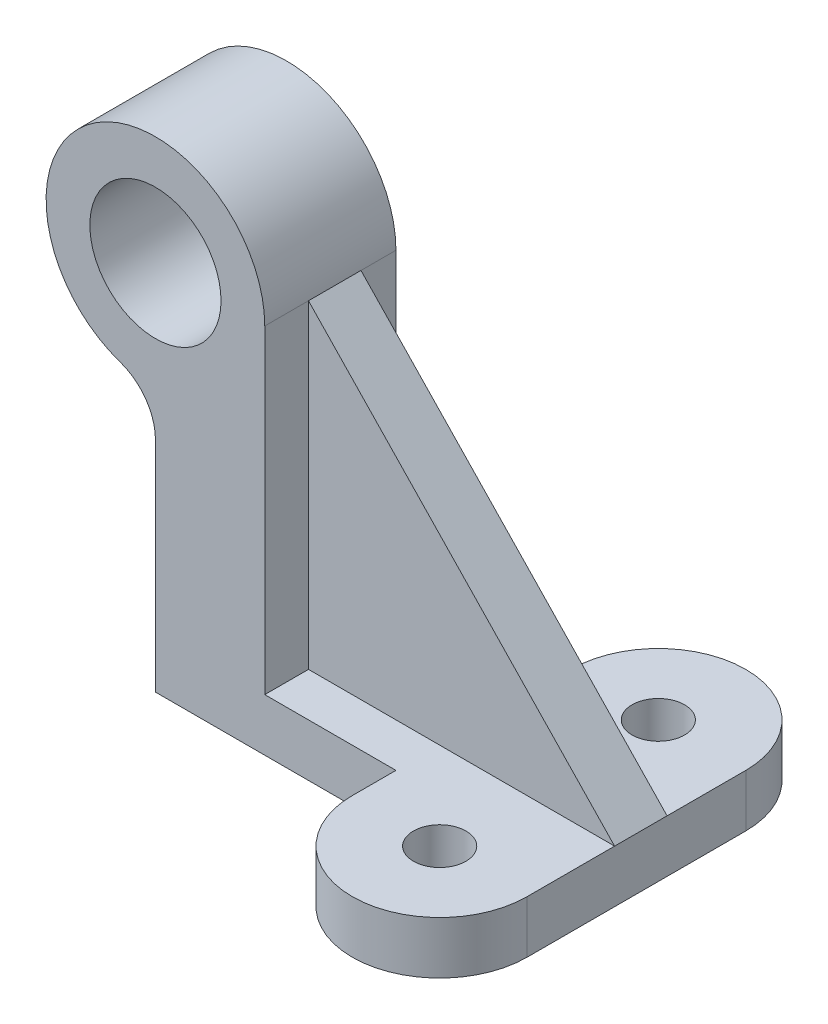
ISO-10303-21;
HEADER;
FILE_DESCRIPTION(('STEP AP214'),'2;1');
FILE_NAME('part.step','',(''),(''),'','','');
FILE_SCHEMA(('AUTOMOTIVE_DESIGN { 1 0 10303 214 1 1 1 1 }'));
ENDSEC;
DATA;
#1=APPLICATION_CONTEXT('core data for automotive mechanical design processes');
#2=APPLICATION_PROTOCOL_DEFINITION('international standard','automotive_design',2000,#1);
#3=PRODUCT_CONTEXT('',#1,'mechanical');
#4=PRODUCT('Part','Part','',(#3));
#5=PRODUCT_RELATED_PRODUCT_CATEGORY('part','',(#4));
#6=PRODUCT_DEFINITION_FORMATION('','',#4);
#7=PRODUCT_DEFINITION_CONTEXT('part definition',#1,'design');
#8=PRODUCT_DEFINITION('design','',#6,#7);
#9=PRODUCT_DEFINITION_SHAPE('','',#8);
#10=(LENGTH_UNIT() NAMED_UNIT(*) SI_UNIT(.MILLI.,.METRE.));
#11=(NAMED_UNIT(*) PLANE_ANGLE_UNIT() SI_UNIT($,.RADIAN.));
#12=(NAMED_UNIT(*) SI_UNIT($,.STERADIAN.) SOLID_ANGLE_UNIT());
#13=UNCERTAINTY_MEASURE_WITH_UNIT(LENGTH_MEASURE(1.E-05),#10,'distance_accuracy_value','');
#14=(GEOMETRIC_REPRESENTATION_CONTEXT(3) GLOBAL_UNCERTAINTY_ASSIGNED_CONTEXT((#13)) GLOBAL_UNIT_ASSIGNED_CONTEXT((#10,
#11,#12)) REPRESENTATION_CONTEXT('',''));
#15=CARTESIAN_POINT('',(0.,0.,0.));
#16=DIRECTION('',(0.,0.,1.));
#17=DIRECTION('',(1.,0.,0.));
#18=AXIS2_PLACEMENT_3D('',#15,#16,#17);
#19=CARTESIAN_POINT('',(0.,6.,-25.));
#20=DIRECTION('',(0.,1.,0.));
#21=DIRECTION('',(0.,0.,1.));
#22=AXIS2_PLACEMENT_3D('',#19,#20,#21);
#23=PLANE('',#22);
#24=DIRECTION('',(-1.,0.,0.));
#25=VECTOR('',#24,1.);
#26=CARTESIAN_POINT('',(20.,6.00000000000001,-7.));
#27=LINE('',#26,#25);
#28=CARTESIAN_POINT('',(20.,6.,-7.00000000000001));
#29=VERTEX_POINT('',#28);
#30=CARTESIAN_POINT('',(-50.,6.,-7.));
#31=VERTEX_POINT('',#30);
#32=EDGE_CURVE('E295',#29,#31,#27,.T.);
#33=ORIENTED_EDGE('',*,*,#32,.F.);
#34=DIRECTION('',(0.,0.,-1.));
#35=VECTOR('',#34,1.);
#36=CARTESIAN_POINT('',(20.,6.,-25.));
#37=LINE('',#36,#35);
#38=CARTESIAN_POINT('',(20.,6.,-25.));
#39=VERTEX_POINT('',#38);
#40=EDGE_CURVE('E58',#29,#39,#37,.T.);
#41=ORIENTED_EDGE('',*,*,#40,.T.);
#42=CARTESIAN_POINT('',(0.,6.,-25.));
#43=DIRECTION('',(0.,1.,0.));
#44=DIRECTION('',(0.,0.,1.));
#45=AXIS2_PLACEMENT_3D('',#42,#43,#44);
#46=CIRCLE('',#45,20.);
#47=CARTESIAN_POINT('',(-20.,6.,-25.));
#48=VERTEX_POINT('',#47);
#49=EDGE_CURVE('E153',#39,#48,#46,.T.);
#50=ORIENTED_EDGE('',*,*,#49,.T.);
#51=DIRECTION('',(0.,0.,1.));
#52=VECTOR('',#51,1.);
#53=CARTESIAN_POINT('',(-20.,6.,-25.));
#54=LINE('',#53,#52);
#55=CARTESIAN_POINT('',(-20.,6.,-15.));
#56=VERTEX_POINT('',#55);
#57=EDGE_CURVE('E97',#48,#56,#54,.T.);
#58=ORIENTED_EDGE('',*,*,#57,.T.);
#59=DIRECTION('',(-1.,0.,0.));
#60=VECTOR('',#59,1.);
#61=CARTESIAN_POINT('',(-20.,6.,-15.));
#62=LINE('',#61,#60);
#63=CARTESIAN_POINT('',(-50.,6.00000000000001,-15.));
#64=VERTEX_POINT('',#63);
#65=EDGE_CURVE('E170',#56,#64,#62,.T.);
#66=ORIENTED_EDGE('',*,*,#65,.T.);
#67=DIRECTION('',(0.,0.,1.));
#68=VECTOR('',#67,1.);
#69=CARTESIAN_POINT('',(-50.,6.,15.));
#70=LINE('',#69,#68);
#71=EDGE_CURVE('E216',#64,#31,#70,.T.);
#72=ORIENTED_EDGE('',*,*,#71,.T.);
#73=EDGE_LOOP('',(#33,#41,#50,#58,#66,#72));
#74=FACE_BOUND('',#73,.T.);
#75=CARTESIAN_POINT('',(0.,6.,-25.));
#76=DIRECTION('',(0.,1.,0.));
#77=DIRECTION('',(0.,0.,1.));
#78=AXIS2_PLACEMENT_3D('',#75,#76,#77);
#79=CIRCLE('',#78,6.);
#80=CARTESIAN_POINT('',(0.,6.,-19.));
#81=VERTEX_POINT('',#80);
#82=EDGE_CURVE('E141',#81,#81,#79,.T.);
#83=ORIENTED_EDGE('',*,*,#82,.F.);
#84=EDGE_LOOP('',(#83));
#85=FACE_BOUND('',#84,.T.);
#86=ADVANCED_FACE('F43',(#74,#85),#23,.T.);
#87=CARTESIAN_POINT('',(-50.,79.,15.));
#88=DIRECTION('',(-1.,0.,0.));
#89=DIRECTION('',(0.,-1.,0.));
#90=AXIS2_PLACEMENT_3D('',#87,#88,#89);
#91=PLANE('',#90);
#92=DIRECTION('',(0.,0.,-1.));
#93=VECTOR('',#92,1.);
#94=CARTESIAN_POINT('',(-50.,79.,15.));
#95=LINE('',#94,#93);
#96=CARTESIAN_POINT('',(-50.,79.,-7.));
#97=VERTEX_POINT('',#96);
#98=CARTESIAN_POINT('',(-50.,79.,-15.));
#99=VERTEX_POINT('',#98);
#100=EDGE_CURVE('E197',#97,#99,#95,.T.);
#101=ORIENTED_EDGE('',*,*,#100,.F.);
#102=DIRECTION('',(0.,-1.,0.));
#103=VECTOR('',#102,1.);
#104=CARTESIAN_POINT('',(-50.,0.,-7.00000000000001));
#105=LINE('',#104,#103);
#106=EDGE_CURVE('E287',#97,#31,#105,.T.);
#107=ORIENTED_EDGE('',*,*,#106,.T.);
#108=ORIENTED_EDGE('',*,*,#71,.F.);
#109=DIRECTION('',(0.,1.,0.));
#110=VECTOR('',#109,1.);
#111=CARTESIAN_POINT('',(-50.,79.,-15.));
#112=LINE('',#111,#110);
#113=EDGE_CURVE('E281',#64,#99,#112,.T.);
#114=ORIENTED_EDGE('',*,*,#113,.T.);
#115=EDGE_LOOP('',(#101,#107,#108,#114));
#116=FACE_BOUND('',#115,.T.);
#117=ADVANCED_FACE('F285',(#116),#91,.F.);
#118=DIRECTION('',(-1.,0.,0.));
#119=VECTOR('',#118,1.);
#120=CARTESIAN_POINT('',(20.,6.00000000000001,5.));
#121=LINE('',#120,#119);
#122=CARTESIAN_POINT('',(20.,6.,5.));
#123=VERTEX_POINT('',#122);
#124=CARTESIAN_POINT('',(-50.,6.,5.));
#125=VERTEX_POINT('',#124);
#126=EDGE_CURVE('E221',#123,#125,#121,.T.);
#127=ORIENTED_EDGE('',*,*,#126,.T.);
#128=CARTESIAN_POINT('',(-50.,6.00000000000001,15.));
#129=VERTEX_POINT('',#128);
#130=EDGE_CURVE('E214',#125,#129,#70,.T.);
#131=ORIENTED_EDGE('',*,*,#130,.T.);
#132=DIRECTION('',(1.,0.,0.));
#133=VECTOR('',#132,1.);
#134=CARTESIAN_POINT('',(-20.,6.,15.));
#135=LINE('',#134,#133);
#136=CARTESIAN_POINT('',(-20.,6.,15.));
#137=VERTEX_POINT('',#136);
#138=EDGE_CURVE('E119',#129,#137,#135,.T.);
#139=ORIENTED_EDGE('',*,*,#138,.T.);
#140=DIRECTION('',(0.,0.,1.));
#141=VECTOR('',#140,1.);
#142=CARTESIAN_POINT('',(-20.,6.,25.));
#143=LINE('',#142,#141);
#144=CARTESIAN_POINT('',(-20.,6.,25.));
#145=VERTEX_POINT('',#144);
#146=EDGE_CURVE('E108',#137,#145,#143,.T.);
#147=ORIENTED_EDGE('',*,*,#146,.T.);
#148=CARTESIAN_POINT('',(0.,6.,25.));
#149=DIRECTION('',(0.,1.,0.));
#150=DIRECTION('',(0.,0.,1.));
#151=AXIS2_PLACEMENT_3D('',#148,#149,#150);
#152=CIRCLE('',#151,20.);
#153=CARTESIAN_POINT('',(20.,6.,25.));
#154=VERTEX_POINT('',#153);
#155=EDGE_CURVE('E118',#145,#154,#152,.T.);
#156=ORIENTED_EDGE('',*,*,#155,.T.);
#157=EDGE_CURVE('E134',#154,#123,#37,.T.);
#158=ORIENTED_EDGE('',*,*,#157,.T.);
#159=EDGE_LOOP('',(#127,#131,#139,#147,#156,#158));
#160=FACE_BOUND('',#159,.T.);
#161=CARTESIAN_POINT('',(0.,6.,25.));
#162=DIRECTION('',(0.,1.,0.));
#163=DIRECTION('',(0.,0.,1.));
#164=AXIS2_PLACEMENT_3D('',#161,#162,#163);
#165=CIRCLE('',#164,6.);
#166=CARTESIAN_POINT('',(0.,6.,31.));
#167=VERTEX_POINT('',#166);
#168=EDGE_CURVE('E205',#167,#167,#165,.T.);
#169=ORIENTED_EDGE('',*,*,#168,.F.);
#170=EDGE_LOOP('',(#169));
#171=FACE_BOUND('',#170,.T.);
#172=ADVANCED_FACE('F115',(#160,#171),#23,.T.);
#173=CARTESIAN_POINT('',(0.,-6.,-25.));
#174=DIRECTION('',(0.,1.,0.));
#175=DIRECTION('',(0.,0.,1.));
#176=AXIS2_PLACEMENT_3D('',#173,#174,#175);
#177=PLANE('',#176);
#178=CARTESIAN_POINT('',(0.,-6.,-25.));
#179=DIRECTION('',(0.,1.,0.));
#180=DIRECTION('',(0.,0.,1.));
#181=AXIS2_PLACEMENT_3D('',#178,#179,#180);
#182=CIRCLE('',#181,20.);
#183=CARTESIAN_POINT('',(20.,-6.,-25.));
#184=VERTEX_POINT('',#183);
#185=CARTESIAN_POINT('',(-20.,-6.,-25.));
#186=VERTEX_POINT('',#185);
#187=EDGE_CURVE('E136',#184,#186,#182,.T.);
#188=ORIENTED_EDGE('',*,*,#187,.F.);
#189=DIRECTION('',(0.,0.,-1.));
#190=VECTOR('',#189,1.);
#191=CARTESIAN_POINT('',(20.,-6.,-25.));
#192=LINE('',#191,#190);
#193=CARTESIAN_POINT('',(20.,-6.,25.));
#194=VERTEX_POINT('',#193);
#195=EDGE_CURVE('E93',#194,#184,#192,.T.);
#196=ORIENTED_EDGE('',*,*,#195,.F.);
#197=CARTESIAN_POINT('',(0.,-6.,25.));
#198=DIRECTION('',(0.,1.,0.));
#199=DIRECTION('',(0.,0.,1.));
#200=AXIS2_PLACEMENT_3D('',#197,#198,#199);
#201=CIRCLE('',#200,20.);
#202=CARTESIAN_POINT('',(-20.,-6.,25.));
#203=VERTEX_POINT('',#202);
#204=EDGE_CURVE('E83',#203,#194,#201,.T.);
#205=ORIENTED_EDGE('',*,*,#204,.F.);
#206=DIRECTION('',(0.,0.,1.));
#207=VECTOR('',#206,1.);
#208=CARTESIAN_POINT('',(-20.,-6.,25.));
#209=LINE('',#208,#207);
#210=CARTESIAN_POINT('',(-20.,-6.,15.));
#211=VERTEX_POINT('',#210);
#212=EDGE_CURVE('E130',#211,#203,#209,.T.);
#213=ORIENTED_EDGE('',*,*,#212,.F.);
#214=DIRECTION('',(1.,0.,0.));
#215=VECTOR('',#214,1.);
#216=CARTESIAN_POINT('',(-20.,-6.,15.));
#217=LINE('',#216,#215);
#218=CARTESIAN_POINT('',(-75.,-6.,15.));
#219=VERTEX_POINT('',#218);
#220=EDGE_CURVE('E146',#219,#211,#217,.T.);
#221=ORIENTED_EDGE('',*,*,#220,.F.);
#222=DIRECTION('',(0.,0.,-1.));
#223=VECTOR('',#222,1.);
#224=CARTESIAN_POINT('',(-75.,-6.,15.));
#225=LINE('',#224,#223);
#226=CARTESIAN_POINT('',(-75.,-6.,-15.));
#227=VERTEX_POINT('',#226);
#228=EDGE_CURVE('E172',#219,#227,#225,.T.);
#229=ORIENTED_EDGE('',*,*,#228,.T.);
#230=DIRECTION('',(-1.,0.,0.));
#231=VECTOR('',#230,1.);
#232=CARTESIAN_POINT('',(-20.,-6.,-15.));
#233=LINE('',#232,#231);
#234=CARTESIAN_POINT('',(-20.,-6.,-15.));
#235=VERTEX_POINT('',#234);
#236=EDGE_CURVE('E144',#235,#227,#233,.T.);
#237=ORIENTED_EDGE('',*,*,#236,.F.);
#238=DIRECTION('',(0.,0.,1.));
#239=VECTOR('',#238,1.);
#240=CARTESIAN_POINT('',(-20.,-6.,-25.));
#241=LINE('',#240,#239);
#242=EDGE_CURVE('E142',#186,#235,#241,.T.);
#243=ORIENTED_EDGE('',*,*,#242,.F.);
#244=EDGE_LOOP('',(#188,#196,#205,#213,#221,#229,#237,#243));
#245=FACE_BOUND('',#244,.T.);
#246=CARTESIAN_POINT('',(0.,-6.,-25.));
#247=DIRECTION('',(0.,1.,0.));
#248=DIRECTION('',(0.,0.,1.));
#249=AXIS2_PLACEMENT_3D('',#246,#247,#248);
#250=CIRCLE('',#249,6.);
#251=CARTESIAN_POINT('',(0.,-6.,-19.));
#252=VERTEX_POINT('',#251);
#253=EDGE_CURVE('E202',#252,#252,#250,.T.);
#254=ORIENTED_EDGE('',*,*,#253,.T.);
#255=EDGE_LOOP('',(#254));
#256=FACE_BOUND('',#255,.T.);
#257=CARTESIAN_POINT('',(0.,-6.,25.));
#258=DIRECTION('',(0.,1.,0.));
#259=DIRECTION('',(0.,0.,1.));
#260=AXIS2_PLACEMENT_3D('',#257,#258,#259);
#261=CIRCLE('',#260,6.);
#262=CARTESIAN_POINT('',(0.,-6.,31.));
#263=VERTEX_POINT('',#262);
#264=EDGE_CURVE('E203',#263,#263,#261,.T.);
#265=ORIENTED_EDGE('',*,*,#264,.T.);
#266=EDGE_LOOP('',(#265));
#267=FACE_BOUND('',#266,.T.);
#268=ADVANCED_FACE('F173',(#245,#256,#267),#177,.F.);
#269=CARTESIAN_POINT('',(0.,6.,-25.));
#270=DIRECTION('',(0.,-1.,0.));
#271=DIRECTION('',(0.,0.,-1.));
#272=AXIS2_PLACEMENT_3D('',#269,#270,#271);
#273=CYLINDRICAL_SURFACE('',#272,20.);
#274=ORIENTED_EDGE('',*,*,#187,.T.);
#275=DIRECTION('',(0.,-1.,0.));
#276=VECTOR('',#275,1.);
#277=CARTESIAN_POINT('',(-20.,6.,-25.));
#278=LINE('',#277,#276);
#279=EDGE_CURVE('E11',#48,#186,#278,.T.);
#280=ORIENTED_EDGE('',*,*,#279,.F.);
#281=ORIENTED_EDGE('',*,*,#49,.F.);
#282=DIRECTION('',(0.,-1.,0.));
#283=VECTOR('',#282,1.);
#284=CARTESIAN_POINT('',(20.,6.,-25.));
#285=LINE('',#284,#283);
#286=EDGE_CURVE('E139',#39,#184,#285,.T.);
#287=ORIENTED_EDGE('',*,*,#286,.T.);
#288=EDGE_LOOP('',(#274,#280,#281,#287));
#289=FACE_BOUND('',#288,.T.);
#290=ADVANCED_FACE('F44',(#289),#273,.T.);
#291=CARTESIAN_POINT('',(-20.,6.,-25.));
#292=DIRECTION('',(1.,0.,0.));
#293=DIRECTION('',(0.,0.,-1.));
#294=AXIS2_PLACEMENT_3D('',#291,#292,#293);
#295=PLANE('',#294);
#296=ORIENTED_EDGE('',*,*,#242,.T.);
#297=DIRECTION('',(0.,-1.,0.));
#298=VECTOR('',#297,1.);
#299=CARTESIAN_POINT('',(-20.,6.,-15.));
#300=LINE('',#299,#298);
#301=EDGE_CURVE('E55',#56,#235,#300,.T.);
#302=ORIENTED_EDGE('',*,*,#301,.F.);
#303=ORIENTED_EDGE('',*,*,#57,.F.);
#304=ORIENTED_EDGE('',*,*,#279,.T.);
#305=EDGE_LOOP('',(#296,#302,#303,#304));
#306=FACE_BOUND('',#305,.T.);
#307=ADVANCED_FACE('F327',(#306),#295,.F.);
#308=CARTESIAN_POINT('',(-20.,6.,-15.));
#309=DIRECTION('',(0.,0.,1.));
#310=DIRECTION('',(1.,0.,0.));
#311=AXIS2_PLACEMENT_3D('',#308,#309,#310);
#312=PLANE('',#311);
#313=ORIENTED_EDGE('',*,*,#236,.T.);
#314=DIRECTION('',(0.,-1.,0.));
#315=VECTOR('',#314,1.);
#316=CARTESIAN_POINT('',(-75.,-6.,-15.));
#317=LINE('',#316,#315);
#318=CARTESIAN_POINT('',(-75.,44.,-15.));
#319=VERTEX_POINT('',#318);
#320=EDGE_CURVE('E195',#319,#227,#317,.T.);
#321=ORIENTED_EDGE('',*,*,#320,.F.);
#322=CARTESIAN_POINT('',(-87.,44.,-15.));
#323=DIRECTION('',(0.,0.,-1.));
#324=DIRECTION('',(1.,0.,0.));
#325=AXIS2_PLACEMENT_3D('',#322,#323,#324);
#326=CIRCLE('',#325,12.);
#327=CARTESIAN_POINT('',(-83.1081081081081,55.3513513513514,-15.));
#328=VERTEX_POINT('',#327);
#329=EDGE_CURVE('E498',#328,#319,#326,.T.);
#330=ORIENTED_EDGE('',*,*,#329,.F.);
#331=CARTESIAN_POINT('',(-75.,79.,-15.));
#332=DIRECTION('',(0.,0.,1.));
#333=DIRECTION('',(1.,0.,0.));
#334=AXIS2_PLACEMENT_3D('',#331,#332,#333);
#335=CIRCLE('',#334,25.);
#336=EDGE_CURVE('E289',#99,#328,#335,.T.);
#337=ORIENTED_EDGE('',*,*,#336,.F.);
#338=ORIENTED_EDGE('',*,*,#113,.F.);
#339=ORIENTED_EDGE('',*,*,#65,.F.);
#340=ORIENTED_EDGE('',*,*,#301,.T.);
#341=EDGE_LOOP('',(#313,#321,#330,#337,#338,#339,#340));
#342=FACE_BOUND('',#341,.T.);
#343=CARTESIAN_POINT('',(-75.,79.,-15.));
#344=DIRECTION('',(0.,0.,1.));
#345=DIRECTION('',(1.,0.,0.));
#346=AXIS2_PLACEMENT_3D('',#343,#344,#345);
#347=CIRCLE('',#346,15.);
#348=CARTESIAN_POINT('',(-60.,79.,-15.));
#349=VERTEX_POINT('',#348);
#350=EDGE_CURVE('E492',#349,#349,#347,.T.);
#351=ORIENTED_EDGE('',*,*,#350,.T.);
#352=EDGE_LOOP('',(#351));
#353=FACE_BOUND('',#352,.T.);
#354=ADVANCED_FACE('F159',(#342,#353),#312,.F.);
#355=CARTESIAN_POINT('',(-20.,6.,15.));
#356=DIRECTION('',(0.,0.,-1.));
#357=DIRECTION('',(-1.,0.,0.));
#358=AXIS2_PLACEMENT_3D('',#355,#356,#357);
#359=PLANE('',#358);
#360=ORIENTED_EDGE('',*,*,#220,.T.);
#361=DIRECTION('',(0.,-1.,0.));
#362=VECTOR('',#361,1.);
#363=CARTESIAN_POINT('',(-20.,6.,15.));
#364=LINE('',#363,#362);
#365=EDGE_CURVE('E126',#137,#211,#364,.T.);
#366=ORIENTED_EDGE('',*,*,#365,.F.);
#367=ORIENTED_EDGE('',*,*,#138,.F.);
#368=DIRECTION('',(0.,1.,0.));
#369=VECTOR('',#368,1.);
#370=CARTESIAN_POINT('',(-50.,79.,15.));
#371=LINE('',#370,#369);
#372=CARTESIAN_POINT('',(-50.,79.,15.));
#373=VERTEX_POINT('',#372);
#374=EDGE_CURVE('E227',#129,#373,#371,.T.);
#375=ORIENTED_EDGE('',*,*,#374,.T.);
#376=CARTESIAN_POINT('',(-75.,79.,15.));
#377=DIRECTION('',(0.,0.,1.));
#378=DIRECTION('',(1.,0.,0.));
#379=AXIS2_PLACEMENT_3D('',#376,#377,#378);
#380=CIRCLE('',#379,25.);
#381=CARTESIAN_POINT('',(-83.1081081081081,55.3513513513514,15.));
#382=VERTEX_POINT('',#381);
#383=EDGE_CURVE('E233',#373,#382,#380,.T.);
#384=ORIENTED_EDGE('',*,*,#383,.T.);
#385=CARTESIAN_POINT('',(-87.,44.,15.));
#386=DIRECTION('',(0.,0.,-1.));
#387=DIRECTION('',(1.,0.,0.));
#388=AXIS2_PLACEMENT_3D('',#385,#386,#387);
#389=CIRCLE('',#388,12.);
#390=CARTESIAN_POINT('',(-75.,44.,15.));
#391=VERTEX_POINT('',#390);
#392=EDGE_CURVE('E189',#382,#391,#389,.T.);
#393=ORIENTED_EDGE('',*,*,#392,.T.);
#394=DIRECTION('',(0.,-1.,0.));
#395=VECTOR('',#394,1.);
#396=CARTESIAN_POINT('',(-75.,-6.,15.));
#397=LINE('',#396,#395);
#398=EDGE_CURVE('E184',#391,#219,#397,.T.);
#399=ORIENTED_EDGE('',*,*,#398,.T.);
#400=EDGE_LOOP('',(#360,#366,#367,#375,#384,#393,#399));
#401=FACE_BOUND('',#400,.T.);
#402=CARTESIAN_POINT('',(-75.,79.,15.));
#403=DIRECTION('',(0.,0.,1.));
#404=DIRECTION('',(1.,0.,0.));
#405=AXIS2_PLACEMENT_3D('',#402,#403,#404);
#406=CIRCLE('',#405,15.);
#407=CARTESIAN_POINT('',(-60.,79.,15.));
#408=VERTEX_POINT('',#407);
#409=EDGE_CURVE('E286',#408,#408,#406,.T.);
#410=ORIENTED_EDGE('',*,*,#409,.F.);
#411=EDGE_LOOP('',(#410));
#412=FACE_BOUND('',#411,.T.);
#413=ADVANCED_FACE('F240',(#401,#412),#359,.F.);
#414=CARTESIAN_POINT('',(-20.,6.,25.));
#415=DIRECTION('',(1.,0.,0.));
#416=DIRECTION('',(0.,0.,-1.));
#417=AXIS2_PLACEMENT_3D('',#414,#415,#416);
#418=PLANE('',#417);
#419=ORIENTED_EDGE('',*,*,#212,.T.);
#420=DIRECTION('',(0.,-1.,0.));
#421=VECTOR('',#420,1.);
#422=CARTESIAN_POINT('',(-20.,6.,25.));
#423=LINE('',#422,#421);
#424=EDGE_CURVE('E121',#145,#203,#423,.T.);
#425=ORIENTED_EDGE('',*,*,#424,.F.);
#426=ORIENTED_EDGE('',*,*,#146,.F.);
#427=ORIENTED_EDGE('',*,*,#365,.T.);
#428=EDGE_LOOP('',(#419,#425,#426,#427));
#429=FACE_BOUND('',#428,.T.);
#430=ADVANCED_FACE('F123',(#429),#418,.F.);
#431=CARTESIAN_POINT('',(0.,6.,25.));
#432=DIRECTION('',(0.,-1.,0.));
#433=DIRECTION('',(0.,0.,-1.));
#434=AXIS2_PLACEMENT_3D('',#431,#432,#433);
#435=CYLINDRICAL_SURFACE('',#434,20.);
#436=ORIENTED_EDGE('',*,*,#204,.T.);
#437=DIRECTION('',(0.,-1.,0.));
#438=VECTOR('',#437,1.);
#439=CARTESIAN_POINT('',(20.,6.,25.));
#440=LINE('',#439,#438);
#441=EDGE_CURVE('E129',#154,#194,#440,.T.);
#442=ORIENTED_EDGE('',*,*,#441,.F.);
#443=ORIENTED_EDGE('',*,*,#155,.F.);
#444=ORIENTED_EDGE('',*,*,#424,.T.);
#445=EDGE_LOOP('',(#436,#442,#443,#444));
#446=FACE_BOUND('',#445,.T.);
#447=ADVANCED_FACE('F133',(#446),#435,.T.);
#448=CARTESIAN_POINT('',(20.,6.,-25.));
#449=DIRECTION('',(-1.,0.,0.));
#450=DIRECTION('',(0.,0.,1.));
#451=AXIS2_PLACEMENT_3D('',#448,#449,#450);
#452=PLANE('',#451);
#453=ORIENTED_EDGE('',*,*,#40,.F.);
#454=DIRECTION('',(0.,0.,1.));
#455=VECTOR('',#454,1.);
#456=CARTESIAN_POINT('',(20.,6.,-65.));
#457=LINE('',#456,#455);
#458=EDGE_CURVE('E250',#29,#123,#457,.T.);
#459=ORIENTED_EDGE('',*,*,#458,.T.);
#460=ORIENTED_EDGE('',*,*,#157,.F.);
#461=ORIENTED_EDGE('',*,*,#441,.T.);
#462=ORIENTED_EDGE('',*,*,#195,.T.);
#463=ORIENTED_EDGE('',*,*,#286,.F.);
#464=EDGE_LOOP('',(#453,#459,#460,#461,#462,#463));
#465=FACE_BOUND('',#464,.T.);
#466=ADVANCED_FACE('F245',(#465),#452,.F.);
#467=CARTESIAN_POINT('',(0.,6.,-25.));
#468=DIRECTION('',(0.,-1.,0.));
#469=DIRECTION('',(0.,0.,-1.));
#470=AXIS2_PLACEMENT_3D('',#467,#468,#469);
#471=CYLINDRICAL_SURFACE('',#470,6.);
#472=ORIENTED_EDGE('',*,*,#82,.T.);
#473=EDGE_LOOP('',(#472));
#474=FACE_BOUND('',#473,.T.);
#475=ORIENTED_EDGE('',*,*,#253,.F.);
#476=EDGE_LOOP('',(#475));
#477=FACE_BOUND('',#476,.T.);
#478=ADVANCED_FACE('F300',(#474,#477),#471,.F.);
#479=CARTESIAN_POINT('',(0.,6.,25.));
#480=DIRECTION('',(0.,-1.,0.));
#481=DIRECTION('',(0.,0.,-1.));
#482=AXIS2_PLACEMENT_3D('',#479,#480,#481);
#483=CYLINDRICAL_SURFACE('',#482,6.);
#484=ORIENTED_EDGE('',*,*,#168,.T.);
#485=EDGE_LOOP('',(#484));
#486=FACE_BOUND('',#485,.T.);
#487=ORIENTED_EDGE('',*,*,#264,.F.);
#488=EDGE_LOOP('',(#487));
#489=FACE_BOUND('',#488,.T.);
#490=ADVANCED_FACE('F297',(#486,#489),#483,.F.);
#491=ORIENTED_EDGE('',*,*,#130,.F.);
#492=DIRECTION('',(0.,1.,0.));
#493=VECTOR('',#492,1.);
#494=CARTESIAN_POINT('',(-50.,0.,5.));
#495=LINE('',#494,#493);
#496=CARTESIAN_POINT('',(-50.,79.,5.));
#497=VERTEX_POINT('',#496);
#498=EDGE_CURVE('E490',#125,#497,#495,.T.);
#499=ORIENTED_EDGE('',*,*,#498,.T.);
#500=EDGE_CURVE('E196',#373,#497,#95,.T.);
#501=ORIENTED_EDGE('',*,*,#500,.F.);
#502=ORIENTED_EDGE('',*,*,#374,.F.);
#503=EDGE_LOOP('',(#491,#499,#501,#502));
#504=FACE_BOUND('',#503,.T.);
#505=ADVANCED_FACE('F232',(#504),#91,.F.);
#506=CARTESIAN_POINT('',(-75.,79.,15.));
#507=DIRECTION('',(0.,0.,-1.));
#508=DIRECTION('',(-1.,0.,0.));
#509=AXIS2_PLACEMENT_3D('',#506,#507,#508);
#510=CYLINDRICAL_SURFACE('',#509,25.);
#511=ORIENTED_EDGE('',*,*,#336,.T.);
#512=DIRECTION('',(0.,0.,-1.));
#513=VECTOR('',#512,1.);
#514=CARTESIAN_POINT('',(-83.1081081081081,55.3513513513514,15.));
#515=LINE('',#514,#513);
#516=EDGE_CURVE('E190',#382,#328,#515,.T.);
#517=ORIENTED_EDGE('',*,*,#516,.F.);
#518=ORIENTED_EDGE('',*,*,#383,.F.);
#519=ORIENTED_EDGE('',*,*,#500,.T.);
#520=DIRECTION('',(0.,0.,1.));
#521=VECTOR('',#520,1.);
#522=CARTESIAN_POINT('',(-50.,79.,0.));
#523=LINE('',#522,#521);
#524=EDGE_CURVE('E483',#97,#497,#523,.T.);
#525=ORIENTED_EDGE('',*,*,#524,.F.);
#526=ORIENTED_EDGE('',*,*,#100,.T.);
#527=EDGE_LOOP('',(#511,#517,#518,#519,#525,#526));
#528=FACE_BOUND('',#527,.T.);
#529=ADVANCED_FACE('F314',(#528),#510,.T.);
#530=CARTESIAN_POINT('',(-87.,44.,15.));
#531=DIRECTION('',(0.,0.,-1.));
#532=DIRECTION('',(-1.,0.,0.));
#533=AXIS2_PLACEMENT_3D('',#530,#531,#532);
#534=CYLINDRICAL_SURFACE('',#533,12.);
#535=ORIENTED_EDGE('',*,*,#329,.T.);
#536=DIRECTION('',(0.,0.,-1.));
#537=VECTOR('',#536,1.);
#538=CARTESIAN_POINT('',(-75.,44.,15.));
#539=LINE('',#538,#537);
#540=EDGE_CURVE('E181',#391,#319,#539,.T.);
#541=ORIENTED_EDGE('',*,*,#540,.F.);
#542=ORIENTED_EDGE('',*,*,#392,.F.);
#543=ORIENTED_EDGE('',*,*,#516,.T.);
#544=EDGE_LOOP('',(#535,#541,#542,#543));
#545=FACE_BOUND('',#544,.T.);
#546=ADVANCED_FACE('F403',(#545),#534,.F.);
#547=CARTESIAN_POINT('',(-75.,-6.,15.));
#548=DIRECTION('',(1.,0.,0.));
#549=DIRECTION('',(0.,0.,-1.));
#550=AXIS2_PLACEMENT_3D('',#547,#548,#549);
#551=PLANE('',#550);
#552=ORIENTED_EDGE('',*,*,#320,.T.);
#553=ORIENTED_EDGE('',*,*,#228,.F.);
#554=ORIENTED_EDGE('',*,*,#398,.F.);
#555=ORIENTED_EDGE('',*,*,#540,.T.);
#556=EDGE_LOOP('',(#552,#553,#554,#555));
#557=FACE_BOUND('',#556,.T.);
#558=ADVANCED_FACE('F409',(#557),#551,.F.);
#559=CARTESIAN_POINT('',(-75.,79.,15.));
#560=DIRECTION('',(0.,0.,-1.));
#561=DIRECTION('',(-1.,0.,0.));
#562=AXIS2_PLACEMENT_3D('',#559,#560,#561);
#563=CYLINDRICAL_SURFACE('',#562,15.);
#564=ORIENTED_EDGE('',*,*,#409,.T.);
#565=EDGE_LOOP('',(#564));
#566=FACE_BOUND('',#565,.T.);
#567=ORIENTED_EDGE('',*,*,#350,.F.);
#568=EDGE_LOOP('',(#567));
#569=FACE_BOUND('',#568,.T.);
#570=ADVANCED_FACE('F420',(#566,#569),#563,.F.);
#571=CARTESIAN_POINT('',(20.,0.,-7.00000000000001));
#572=DIRECTION('',(0.,0.,-1.));
#573=DIRECTION('',(0.,1.,0.));
#574=AXIS2_PLACEMENT_3D('',#571,#572,#573);
#575=PLANE('',#574);
#576=DIRECTION('',(-0.692120082233928,0.721782371472524,0.));
#577=VECTOR('',#576,1.);
#578=CARTESIAN_POINT('',(22.9973604457914,2.874181249389,-7.00000000000001));
#579=LINE('',#578,#577);
#580=EDGE_CURVE('E481',#29,#97,#579,.T.);
#581=ORIENTED_EDGE('',*,*,#580,.F.);
#582=ORIENTED_EDGE('',*,*,#32,.T.);
#583=ORIENTED_EDGE('',*,*,#106,.F.);
#584=EDGE_LOOP('',(#581,#582,#583));
#585=FACE_BOUND('',#584,.T.);
#586=ADVANCED_FACE('F426',(#585),#575,.T.);
#587=CARTESIAN_POINT('',(20.,0.,5.));
#588=DIRECTION('',(0.,0.,1.));
#589=DIRECTION('',(1.,0.,0.));
#590=AXIS2_PLACEMENT_3D('',#587,#588,#589);
#591=PLANE('',#590);
#592=DIRECTION('',(0.692120082233928,-0.721782371472524,0.));
#593=VECTOR('',#592,1.);
#594=CARTESIAN_POINT('',(20.,6.,5.));
#595=LINE('',#594,#593);
#596=EDGE_CURVE('E506',#497,#123,#595,.T.);
#597=ORIENTED_EDGE('',*,*,#596,.F.);
#598=ORIENTED_EDGE('',*,*,#498,.F.);
#599=ORIENTED_EDGE('',*,*,#126,.F.);
#600=EDGE_LOOP('',(#597,#598,#599));
#601=FACE_BOUND('',#600,.T.);
#602=ADVANCED_FACE('F456',(#601),#591,.T.);
#603=CARTESIAN_POINT('',(20.,6.,-65.));
#604=DIRECTION('',(-0.721782371472524,-0.692120082233928,0.));
#605=DIRECTION('',(0.692120082233928,-0.721782371472524,0.));
#606=AXIS2_PLACEMENT_3D('',#603,#604,#605);
#607=PLANE('',#606);
#608=ORIENTED_EDGE('',*,*,#580,.T.);
#609=ORIENTED_EDGE('',*,*,#524,.T.);
#610=ORIENTED_EDGE('',*,*,#596,.T.);
#611=ORIENTED_EDGE('',*,*,#458,.F.);
#612=EDGE_LOOP('',(#608,#609,#610,#611));
#613=FACE_BOUND('',#612,.T.);
#614=ADVANCED_FACE('F467',(#613),#607,.F.);
#615=CLOSED_SHELL('',(#86,#117,#172,#268,#290,#307,#354,#413,#430,#447,#466,#478,#490,#505,#529,
#546,#558,#570,#586,#602,#614));
#616=MANIFOLD_SOLID_BREP('B2',#615);
#617=ADVANCED_BREP_SHAPE_REPRESENTATION('',(#18,#616),#14);
#618=SHAPE_DEFINITION_REPRESENTATION(#9,#617);
ENDSEC;
END-ISO-10303-21;
